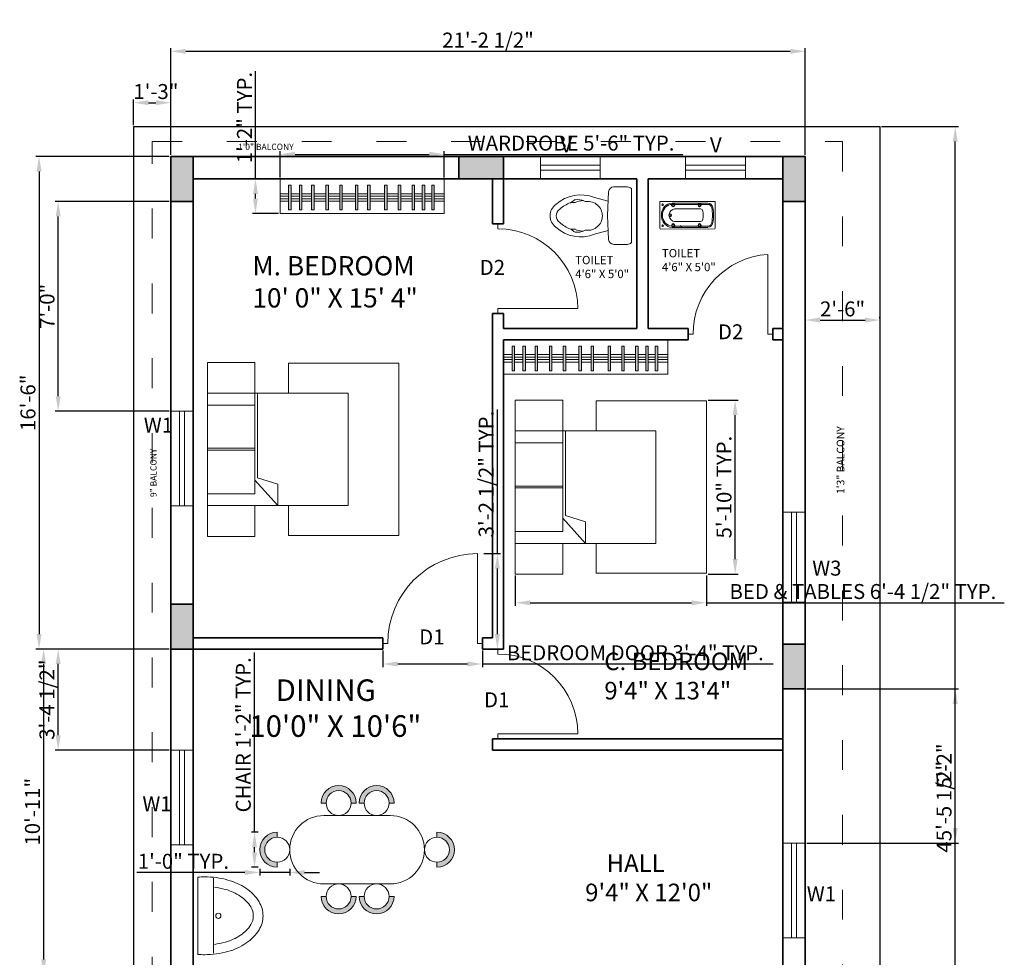
# Model space of a CAD drawing. Units: inches. Extents: x 40559 to 41508, y 131086 to 132358.
# Tile 2 of 5: x 40559 to 40954, y 131334 to 131710. Entities that reach past the tile are written whole.
import ezdxf

# ---------------------------------------------------------------- set-up
doc = ezdxf.new("R2010")
doc.units = ezdxf.units.IN
doc.linetypes.add('ACAD_ISO03W100', pattern=[30, 12, -18])
for name, color, linetype, lineweight in [('A-ANNO-DIMS', 2, 'Continuous', 18), ('A-ANNO-TEXT', 7, 'Continuous', 18), ('A-AREA-IDEN', 7, 'Continuous', 18), ('A-FLOR-FIXT', 4, 'Continuous', 18), ('A-FLOR-OVHD', 240, 'ACAD_ISO03W100', 13), ('A-FURN', 9, 'Continuous', 18), ('A-FURN-PATT', 252, 'Continuous', 13), ('A-WALL', 7, 'Continuous', 35), ('C-PROP', 7, 'Continuous', 25), ('Doors', 50, 'Continuous', 18), ('Windows', 70, 'Continuous', 18)]:
    doc.layers.add(name, color=color, linetype=linetype, lineweight=lineweight)
doc.layers.add('A-COLS', color=177, linetype='Continuous', lineweight=35, true_color=0x293189)
doc.styles.get("Standard").update_dxf_attribs({"font": 'arial.ttf'})
doc.dimstyles.new('ISO-25', dxfattribs={"dimtxt": 6, "dimasz": 6, "dimexe": 1.25, "dimexo": 0.625, "dimtad": 1, "dimdec": 0, "dimlunit": 3, "dimtxsty": 'Standard', "dimcen": 2.5, "dimclrd": 1, "dimclre": 1, "dimclrt": 2, "dimadec": 0, "dimazin": 0, "dimtfac": 1, "dimtdec": 0, "dimtmove": 0, "dimatfit": 3, "dimfxl": 1, "dimarcsym": 0})

# ---------------------------------------------------------------- blocks, each defined once
blk = doc.blocks.new('*D8')
at = {"layer": 'A-ANNO-DIMS', "color": 0, "lineweight": -2, "transparency": 16777216}
for p, q in [((40604.44, 131667.98), (40604.44, 131678.2)), ((40610.44, 131676.95), (40613.44, 131676.95)), ((40619.44, 131667.98), (40619.44, 131678.2))]:
    blk.add_line(p, q, dxfattribs=at)
at = {"layer": 'A-ANNO-DIMS', "color": 0, "transparency": 16777216}
for points in [[(40610.44, 131677.95), (40610.44, 131675.95), (40604.44, 131676.95)], [(40613.44, 131677.95), (40613.44, 131675.95), (40619.44, 131676.95)]]:
    blk.add_solid(points, dxfattribs=at)
at = {"layer": 'Defpoints', "color": 0, "transparency": 16777216}
for p in [(40619.44, 131676.95), (40604.44, 131667.35), (40619.44, 131667.35)]:
    blk.add_point(p, dxfattribs=at)
at = {"layer": 'A-ANNO-DIMS', "color": 0, "transparency": 16777216, "insert": (40613.44, 131680.64), "char_height": 6, "attachment_point": 5}
blk.add_mtext('1\'-3"', dxfattribs=at)
blk = doc.blocks.new('*D9')
at = {"layer": 'A-ANNO-DIMS', "color": 0, "lineweight": -2, "transparency": 16777216}
for p, q in [((40618.81, 131655.35), (40565.32, 131655.35)), ((40566.57, 131649.35), (40566.57, 131463.85)), ((40618.81, 131457.85), (40565.32, 131457.85))]:
    blk.add_line(p, q, dxfattribs=at)
at = {"layer": 'A-ANNO-DIMS', "color": 0, "transparency": 16777216}
for points in [[(40565.57, 131649.35), (40567.57, 131649.35), (40566.57, 131655.35)], [(40565.57, 131463.85), (40567.57, 131463.85), (40566.57, 131457.85)]]:
    blk.add_solid(points, dxfattribs=at)
at = {"layer": 'Defpoints', "color": 0, "transparency": 16777216}
for p in [(40619.44, 131655.35), (40566.57, 131457.85), (40619.44, 131457.85)]:
    blk.add_point(p, dxfattribs=at)
at = {"layer": 'A-ANNO-DIMS', "color": 0, "transparency": 16777216, "insert": (40562.88, 131556.6), "char_height": 6, "attachment_point": 5, "rotation": 90}
blk.add_mtext('16\'-6"', dxfattribs=at)
blk = doc.blocks.new('*D10')
at = {"layer": 'A-ANNO-DIMS', "color": 0, "lineweight": -2, "transparency": 16777216}
for p, q in [((40618.81, 131457.85), (40567.14, 131457.85)), ((40568.39, 131451.85), (40568.39, 131333.35)), ((40627.81, 131327.35), (40567.14, 131327.35))]:
    blk.add_line(p, q, dxfattribs=at)
at = {"layer": 'A-ANNO-DIMS', "color": 0, "transparency": 16777216}
for points in [[(40567.39, 131451.85), (40569.39, 131451.85), (40568.39, 131457.85)], [(40567.39, 131333.35), (40569.39, 131333.35), (40568.39, 131327.35)]]:
    blk.add_solid(points, dxfattribs=at)
at = {"layer": 'Defpoints', "color": 0, "transparency": 16777216}
for p in [(40619.44, 131457.85), (40568.39, 131327.35), (40628.44, 131327.35)]:
    blk.add_point(p, dxfattribs=at)
at = {"layer": 'A-ANNO-DIMS', "color": 0, "transparency": 16777216, "insert": (40564.7, 131392.6), "char_height": 6, "attachment_point": 5, "rotation": 90}
blk.add_mtext('10\'-11"', dxfattribs=at)
blk = doc.blocks.new('*D7')
at = {"layer": 'A-ANNO-DIMS', "color": 0, "lineweight": -2, "transparency": 16777216}
for p, q in [((40873.94, 131590.4), (40873.94, 131591.03)), ((40879.94, 131589.78), (40897.94, 131589.78)), ((40903.94, 131590.4), (40903.94, 131591.03))]:
    blk.add_line(p, q, dxfattribs=at)
at = {"layer": 'A-ANNO-DIMS', "color": 0, "transparency": 16777216}
for points in [[(40879.94, 131590.78), (40879.94, 131588.78), (40873.94, 131589.78)], [(40897.94, 131590.78), (40897.94, 131588.78), (40903.94, 131589.78)]]:
    blk.add_solid(points, dxfattribs=at)
at = {"layer": 'Defpoints', "color": 0, "transparency": 16777216}
for p in [(40873.94, 131589.78), (40903.94, 131589.78), (40903.94, 131589.78)]:
    blk.add_point(p, dxfattribs=at)
at = {"layer": 'A-ANNO-DIMS', "color": 0, "transparency": 16777216, "insert": (40888.94, 131593.47), "char_height": 6, "attachment_point": 5}
blk.add_mtext('2\'-6"', dxfattribs=at)
blk = doc.blocks.new('WIN-36IN')
for p, q in [((0, 5.5), (36, 5.5)), ((0, 3.5), (36, 3.5))]:
    blk.add_line(p, q)
blk.add_lwpolyline([(0, 9), (36, 9), (36, 0), (0, 0)], close=True)
blk = doc.blocks.new('WIN-38IN')
for p, q in [((0, 5.5), (38, 5.5)), ((0, 3.5), (38, 3.5))]:
    blk.add_line(p, q)
blk.add_lwpolyline([(0, 9), (38, 9), (38, 0), (0, 0)], close=True)
blk = doc.blocks.new('VENT-24IN')
for p, q in [((0, 5.5), (24, 5.5)), ((0, 3.5), (24, 3.5))]:
    blk.add_line(p, q)
blk.add_lwpolyline([(0, 9), (24, 9), (24, 0), (0, 0)], close=True)
blk = doc.blocks.new('DOOR-INT-36IN')
for p, q in [((2.25, 34), (2.25, 36)), ((4.5, 0), (0, 0)), ((2.25, 0), (2.25, 2)), ((2.25, 2), (34.25, 2))]:
    blk.add_line(p, q)
blk.add_arc((2.25, 2), 32, 0, 90)
blk = doc.blocks.new('DOOR-BATH-34IN')
for p, q in [((32, 2.25), (32, 34.25)), ((34, 4.5), (34, 0)), ((0, 2.25), (2, 2.25)), ((34, 2.25), (32, 2.25))]:
    blk.add_line(p, q)
blk.add_arc((34.07, 2.25), 32.07, 93.6952, 180)
blk = doc.blocks.new('DOOR-INT-40IN')
for p, q in [((38, 2.25), (38, 38.25)), ((40, 4.5), (40, 0)), ((2, 2.25), (0, 2.25)), ((40, 2.25), (38, 2.25))]:
    blk.add_line(p, q)
blk.add_arc((38, 2.25), 36, 90, 180)
blk = doc.blocks.new('COL-9X18IN')
h = blk.add_hatch(color=256)
h.dxf.hatch_style = 1
h.paths.add_polyline_path([(9, 18), (0, 18), (0, 0), (9, 0)])
blk.add_lwpolyline([(0, 18), (9, 18), (9, 0), (0, 0)], close=True)
blk = doc.blocks.new('WARDROBE-PLAN')
h = blk.add_hatch(color=256)
h.dxf.hatch_style = 1
h.paths.add_polyline_path([(4.39, 11.35), (3.39, 11.35), (3.39, 1.43), (4.39, 1.43)])
h.paths.add_polyline_path([(19.37, 11.35), (18.37, 11.35), (18.37, 1.43), (19.37, 1.43)])
h.paths.add_polyline_path([(48.38, 11.35), (47.38, 11.35), (47.38, 1.43), (48.38, 1.43)])
h.paths.add_polyline_path([(61.87, 11.35), (60.87, 11.35), (60.87, 1.43), (61.87, 1.43)])
h = blk.add_hatch(color=256)
h.dxf.hatch_style = 1
h.paths.add_polyline_path([(8.74, 11.35), (7.74, 11.35), (7.74, 1.43), (8.74, 1.43)])
h.paths.add_polyline_path([(36.12, 11.35), (35.12, 11.35), (35.12, 1.43), (36.12, 1.43)])
h.paths.add_polyline_path([(58.05, 11.35), (57.05, 11.35), (57.05, 1.43), (58.05, 1.43)])
h = blk.add_hatch(color=256)
h.dxf.hatch_style = 1
h.paths.add_polyline_path([(13.65, 11.35), (12.65, 11.35), (12.65, 1.43), (13.65, 1.43)])
h.paths.add_polyline_path([(31.22, 11.35), (30.22, 11.35), (30.22, 1.43), (31.22, 1.43)])
h.paths.add_polyline_path([(53.97, 11.35), (52.97, 11.35), (52.97, 1.43), (53.97, 1.43)])
h = blk.add_hatch(color=256)
h.dxf.hatch_style = 1
h.paths.add_polyline_path([(24.95, 11.35), (23.95, 11.35), (23.95, 1.43), (24.95, 1.43)])
h.paths.add_polyline_path([(42.93, 11.35), (41.93, 11.35), (41.93, 1.43), (42.93, 1.43)])
for p, q in [((0, 13.83), (0, 0)), ((65.87, 0), (65.87, 13.83)), ((0, 7.92), (3.39, 7.92)), ((3.39, 11.35), (3.39, 1.43)), ((3.39, 11.35), (4.39, 11.35)), ((4.39, 11.35), (4.39, 1.43)), ((4.39, 7.92), (7.74, 7.92)), ((7.74, 11.35), (7.74, 1.43)), ((7.74, 11.35), (8.74, 11.35)), ((8.74, 11.35), (8.74, 1.43)), ((8.74, 7.92), (12.65, 7.92)), ((12.65, 11.35), (12.65, 1.43)), ((12.65, 11.35), (13.65, 11.35)), ((13.65, 11.35), (13.65, 1.43)), ((13.65, 7.92), (18.37, 7.92)), ((18.37, 11.35), (18.37, 1.43)), ((18.37, 11.35), (19.37, 11.35)), ((19.37, 11.35), (19.37, 1.43)), ((19.37, 7.92), (23.95, 7.92)), ((23.95, 11.35), (23.95, 1.43)), ((23.95, 11.35), (24.95, 11.35)), ((24.95, 11.35), (24.95, 1.43)), ((24.95, 7.92), (30.22, 7.92)), ((30.22, 11.35), (30.22, 1.43)), ((30.22, 11.35), (31.22, 11.35)), ((31.22, 11.35), (31.22, 1.43)), ((31.22, 7.92), (35.12, 7.92)), ((35.12, 11.35), (35.12, 1.43)), ((35.12, 11.35), (36.12, 11.35)), ((36.12, 11.35), (36.12, 1.43)), ((36.12, 7.92), (41.93, 7.92)), ((41.93, 11.35), (41.93, 1.43)), ((41.93, 11.35), (42.93, 11.35)), ((42.93, 11.35), (42.93, 1.43)), ((42.93, 7.92), (47.38, 7.92)), ((47.38, 11.35), (47.38, 1.43)), ((47.38, 11.35), (48.38, 11.35)), ((48.38, 11.35), (48.38, 1.43)), ((48.38, 7.92), (52.97, 7.92)), ((52.97, 11.35), (52.97, 1.43)), ((52.97, 11.35), (53.97, 11.35)), ((53.97, 11.35), (53.97, 1.43)), ((53.97, 7.92), (57.05, 7.92)), ((57.05, 11.35), (57.05, 1.43)), ((57.05, 11.35), (58.05, 11.35)), ((58.05, 11.35), (58.05, 1.43)), ((58.05, 7.92), (60.87, 7.92)), ((60.87, 11.35), (60.87, 1.43)), ((60.87, 11.35), (61.87, 11.35)), ((61.87, 11.35), (61.87, 1.43)), ((61.87, 7.92), (65.87, 7.92)), ((0, 6.92), (3.39, 6.92)), ((0, 5.92), (3.39, 5.92)), ((0, 4.92), (3.39, 4.92)), ((4.39, 6.92), (7.74, 6.92)), ((4.39, 5.92), (7.74, 5.92)), ((4.39, 4.92), (7.74, 4.92)), ((8.74, 6.92), (12.65, 6.92)), ((8.74, 5.92), (12.65, 5.92)), ((8.74, 4.92), (12.65, 4.92)), ((13.65, 6.92), (18.37, 6.92)), ((13.65, 5.92), (18.37, 5.92)), ((13.65, 4.92), (18.37, 4.92)), ((19.37, 6.92), (23.95, 6.92)), ((19.37, 5.92), (23.95, 5.92)), ((19.37, 4.92), (23.95, 4.92)), ((24.95, 6.92), (30.22, 6.92)), ((24.95, 5.92), (30.22, 5.92)), ((24.95, 4.92), (30.22, 4.92)), ((31.22, 6.92), (35.12, 6.92)), ((31.22, 5.92), (35.12, 5.92)), ((31.22, 4.92), (35.12, 4.92)), ((36.12, 6.92), (41.93, 6.92)), ((36.12, 5.92), (41.93, 5.92)), ((36.12, 4.92), (41.93, 4.92)), ((42.93, 6.92), (47.38, 6.92)), ((42.93, 5.92), (47.38, 5.92)), ((42.93, 4.92), (47.38, 4.92)), ((48.38, 6.92), (52.97, 6.92)), ((48.38, 5.92), (52.97, 5.92)), ((48.38, 4.92), (52.97, 4.92)), ((53.97, 6.92), (57.05, 6.92)), ((53.97, 5.92), (57.05, 5.92)), ((53.97, 4.92), (57.05, 4.92)), ((58.05, 6.92), (60.87, 6.92)), ((58.05, 5.92), (60.87, 5.92)), ((58.05, 4.92), (60.87, 4.92)), ((61.87, 6.92), (65.87, 6.92)), ((61.87, 5.92), (65.87, 5.92)), ((61.87, 4.92), (65.87, 4.92)), ((0, 0), (65.87, 0)), ((3.39, 1.43), (4.39, 1.43)), ((7.74, 1.43), (8.74, 1.43)), ((12.65, 1.43), (13.65, 1.43)), ((18.37, 1.43), (19.37, 1.43)), ((23.95, 1.43), (24.95, 1.43)), ((30.22, 1.43), (31.22, 1.43)), ((35.12, 1.43), (36.12, 1.43)), ((41.93, 1.43), (42.93, 1.43)), ((47.38, 1.43), (48.38, 1.43)), ((52.97, 1.43), (53.97, 1.43)), ((57.05, 1.43), (58.05, 1.43)), ((60.87, 1.43), (61.87, 1.43))]:
    blk.add_line(p, q)
blk = doc.blocks.new('BED-WITH-SIDE-TABLES')
for p, q in [((0, 57.45), (0, 69.77)), ((0, 69.77), (19.02, 69.77)), ((19.02, 69.77), (19.02, 57.45)), ((32.44, 57.45), (32.44, 69.45)), ((32.44, 69.45), (76.71, 69.45)), ((76.71, 69.45), (76.71, 0.32)), ((0, 52.63), (0, 57.45)), ((0, 57.45), (56.44, 57.45)), ((19.02, 57.45), (19.02, 22.47)), ((20.12, 23.47), (20.12, 57.45)), ((56.44, 57.45), (56.44, 12.32)), ((0, 52.63), (19.02, 52.63)), ((0, 17.11), (0, 52.63)), ((19.02, 52.63), (19.02, 17.11)), ((0, 35.3), (19.02, 35.3)), ((0, 34.61), (19.02, 34.61)), ((19.02, 22.47), (28.22, 12.32)), ((28.22, 20.94), (20.12, 23.47)), ((28.22, 12.32), (28.22, 20.94)), ((0, 17.11), (19.02, 17.11)), ((0, 17.11), (0, 12.32)), ((0, 12.32), (56.44, 12.32)), ((0, 12.32), (0, 0)), ((19.02, 0), (19.02, 12.32)), ((32.44, 12.32), (32.44, 0.32)), ((0, 0), (19.02, 0)), ((32.44, 0.32), (76.71, 0.32))]:
    blk.add_line(p, q)
blk = doc.blocks.new('DINING-CHAIR')
for p, q in [((1.99, 5.01), (0, 5.01)), ((12.01, 5.01), (13.99, 5.01))]:
    blk.add_line(p, q)
blk.add_circle((7, 5.01), 5.01)
blk.add_arc((7, 5.01), 7, 0, 180)
blk = doc.blocks.new('*D48')
at = {"layer": 'A-ANNO-DIMS', "color": 1, "lineweight": -2, "transparency": 16777216}
for p, q in [((40704.44, 131457.23), (40704.44, 131450.6)), ((40744.44, 131457.23), (40744.44, 131450.6)), ((40710.44, 131451.85), (40738.44, 131451.85)), ((40744.44, 131451.85), (40861.11, 131451.85))]:
    blk.add_line(p, q, dxfattribs=at)
at = {"layer": 'A-ANNO-DIMS', "color": 1, "transparency": 16777216}
for points in [[(40710.44, 131452.85), (40710.44, 131450.85), (40704.44, 131451.85)], [(40738.44, 131452.85), (40738.44, 131450.85), (40744.44, 131451.85)]]:
    blk.add_solid(points, dxfattribs=at)
at = {"layer": 'Defpoints', "color": 0, "transparency": 16777216}
for p in [(40704.44, 131457.85), (40744.44, 131457.85), (40744.44, 131451.85)]:
    blk.add_point(p, dxfattribs=at)
at = {"layer": 'A-ANNO-DIMS', "color": 2, "transparency": 16777216, "insert": (40805.77, 131455.58), "char_height": 6, "attachment_point": 5}
blk.add_mtext('BEDROOM DOOR 3\'-4" TYP.', dxfattribs=at)
blk = doc.blocks.new('*D49')
at = {"layer": 'A-ANNO-DIMS', "color": 1, "lineweight": -2, "transparency": 16777216}
for p, q in [((40750.44, 131496.1), (40750.44, 131553.9)), ((40745.06, 131496.1), (40751.69, 131496.1)), ((40750.44, 131463.85), (40750.44, 131490.1)), ((40745.06, 131457.85), (40751.69, 131457.85))]:
    blk.add_line(p, q, dxfattribs=at)
at = {"layer": 'A-ANNO-DIMS', "color": 1, "transparency": 16777216}
for points in [[(40749.44, 131490.1), (40751.44, 131490.1), (40750.44, 131496.1)], [(40749.44, 131463.85), (40751.44, 131463.85), (40750.44, 131457.85)]]:
    blk.add_solid(points, dxfattribs=at)
at = {"layer": 'Defpoints', "color": 0, "transparency": 16777216}
for p in [(40744.44, 131496.1), (40750.44, 131496.1), (40744.44, 131457.85)]:
    blk.add_point(p, dxfattribs=at)
at = {"layer": 'A-ANNO-DIMS', "color": 2, "transparency": 16777216, "insert": (40746.71, 131528), "char_height": 6, "attachment_point": 5, "rotation": 90}
blk.add_mtext('3\'-2 1/2" TYP.', dxfattribs=at)
blk = doc.blocks.new('*D52')
at = {"layer": 'A-ANNO-DIMS', "color": 1, "lineweight": -2, "transparency": 16777216}
for p, q in [((40653.01, 131384.35), (40653.01, 131456.52)), ((40654.48, 131384.35), (40651.76, 131384.35)), ((40653.01, 131376.36), (40653.01, 131378.35)), ((40654.48, 131370.36), (40651.76, 131370.36))]:
    blk.add_line(p, q, dxfattribs=at)
at = {"layer": 'A-ANNO-DIMS', "color": 1, "transparency": 16777216}
for points in [[(40652.01, 131378.35), (40654.01, 131378.35), (40653.01, 131384.35)], [(40652.01, 131376.36), (40654.01, 131376.36), (40653.01, 131370.36)]]:
    blk.add_solid(points, dxfattribs=at)
at = {"layer": 'Defpoints', "color": 0, "transparency": 16777216}
for p in [(40653.01, 131384.35), (40655.11, 131384.35), (40655.11, 131370.36)]:
    blk.add_point(p, dxfattribs=at)
at = {"layer": 'A-ANNO-DIMS', "color": 2, "transparency": 16777216, "insert": (40649.28, 131423.44), "char_height": 6, "attachment_point": 5, "rotation": 90}
blk.add_mtext('CHAIR 1\'-2" TYP.', dxfattribs=at)
blk = doc.blocks.new('*D53')
at = {"layer": 'A-ANNO-DIMS', "color": 1, "lineweight": -2, "transparency": 16777216}
for p, q in [((40649.11, 131368.26), (40605.85, 131368.26)), ((40655.11, 131369.74), (40655.11, 131367.01)), ((40667.11, 131368.26), (40655.11, 131368.26)), ((40667.11, 131369.74), (40667.11, 131367.01)), ((40673.11, 131368.26), (40679.11, 131368.26))]:
    blk.add_line(p, q, dxfattribs=at)
at = {"layer": 'A-ANNO-DIMS', "color": 1, "transparency": 16777216}
for points in [[(40649.11, 131369.26), (40649.11, 131367.26), (40655.11, 131368.26)], [(40673.11, 131369.26), (40673.11, 131367.26), (40667.11, 131368.26)]]:
    blk.add_solid(points, dxfattribs=at)
at = {"layer": 'Defpoints', "color": 0, "transparency": 16777216}
for p in [(40655.11, 131370.36), (40655.11, 131368.26), (40667.11, 131370.36)]:
    blk.add_point(p, dxfattribs=at)
at = {"layer": 'A-ANNO-DIMS', "color": 2, "transparency": 16777216, "insert": (40624.48, 131371.95), "char_height": 6, "attachment_point": 5}
blk.add_mtext('1\'-0" TYP.', dxfattribs=at)
blk = doc.blocks.new('*D56')
at = {"layer": 'A-ANNO-DIMS', "color": 1, "lineweight": -2, "transparency": 16777216}
for p, q in [((40663.27, 131646.98), (40663.27, 131657.48)), ((40669.27, 131656.23), (40723.14, 131656.23)), ((40729.14, 131646.98), (40729.14, 131657.48)), ((40729.14, 131656.23), (40824.9, 131656.23))]:
    blk.add_line(p, q, dxfattribs=at)
at = {"layer": 'A-ANNO-DIMS', "color": 1, "transparency": 16777216}
for points in [[(40669.27, 131657.23), (40669.27, 131655.23), (40663.27, 131656.23)], [(40723.14, 131657.23), (40723.14, 131655.23), (40729.14, 131656.23)]]:
    blk.add_solid(points, dxfattribs=at)
at = {"layer": 'Defpoints', "color": 0, "transparency": 16777216}
for p in [(40729.14, 131656.23), (40663.27, 131646.35), (40729.14, 131646.35)]:
    blk.add_point(p, dxfattribs=at)
at = {"layer": 'A-ANNO-DIMS', "color": 2, "transparency": 16777216, "insert": (40780.02, 131659.96), "char_height": 6, "attachment_point": 5}
blk.add_mtext('WARDROBE 5\'-6" TYP.', dxfattribs=at)
blk = doc.blocks.new('*D57')
at = {"layer": 'A-ANNO-DIMS', "color": 1, "lineweight": -2, "transparency": 16777216}
for p, q in [((40653.39, 131646.35), (40653.39, 131689.61)), ((40662.64, 131646.35), (40652.14, 131646.35)), ((40653.39, 131638.52), (40653.39, 131640.35)), ((40662.64, 131632.52), (40652.14, 131632.52))]:
    blk.add_line(p, q, dxfattribs=at)
at = {"layer": 'A-ANNO-DIMS', "color": 1, "transparency": 16777216}
for points in [[(40652.39, 131640.35), (40654.39, 131640.35), (40653.39, 131646.35)], [(40652.39, 131638.52), (40654.39, 131638.52), (40653.39, 131632.52)]]:
    blk.add_solid(points, dxfattribs=at)
at = {"layer": 'Defpoints', "color": 0, "transparency": 16777216}
for p in [(40653.39, 131646.35), (40663.27, 131646.35), (40663.27, 131632.52)]:
    blk.add_point(p, dxfattribs=at)
at = {"layer": 'A-ANNO-DIMS', "color": 2, "transparency": 16777216, "insert": (40649.75, 131670.98), "char_height": 6, "attachment_point": 5, "rotation": 90}
blk.add_mtext('1\'-2" TYP.', dxfattribs=at)
blk = doc.blocks.new('*D58')
at = {"layer": 'A-ANNO-DIMS', "color": 1, "lineweight": -2, "transparency": 16777216}
for p, q in [((40757.62, 131487.28), (40757.62, 131475.15)), ((40834.33, 131487.28), (40834.33, 131475.15)), ((40763.62, 131476.4), (40828.33, 131476.4)), ((40834.33, 131476.4), (40953.83, 131476.4))]:
    blk.add_line(p, q, dxfattribs=at)
at = {"layer": 'A-ANNO-DIMS', "color": 1, "transparency": 16777216}
for points in [[(40763.62, 131477.4), (40763.62, 131475.4), (40757.62, 131476.4)], [(40828.33, 131477.4), (40828.33, 131475.4), (40834.33, 131476.4)]]:
    blk.add_solid(points, dxfattribs=at)
at = {"layer": 'Defpoints', "color": 0, "transparency": 16777216}
for p in [(40757.62, 131487.9), (40834.33, 131487.9), (40834.33, 131476.4)]:
    blk.add_point(p, dxfattribs=at)
at = {"layer": 'A-ANNO-DIMS', "color": 2, "transparency": 16777216, "insert": (40897.08, 131480.14), "char_height": 6, "attachment_point": 5}
blk.add_mtext('BED & TABLES 6\'-4 1/2" TYP.', dxfattribs=at)
blk = doc.blocks.new('*D59')
at = {"layer": 'A-ANNO-DIMS', "color": 1, "lineweight": -2, "transparency": 16777216}
for p, q in [((40834.96, 131557.68), (40847.09, 131557.68)), ((40845.84, 131493.9), (40845.84, 131551.68)), ((40834.96, 131487.9), (40847.09, 131487.9))]:
    blk.add_line(p, q, dxfattribs=at)
at = {"layer": 'A-ANNO-DIMS', "color": 1, "transparency": 16777216}
for points in [[(40844.84, 131551.68), (40846.84, 131551.68), (40845.84, 131557.68)], [(40844.84, 131493.9), (40846.84, 131493.9), (40845.84, 131487.9)]]:
    blk.add_solid(points, dxfattribs=at)
at = {"layer": 'Defpoints', "color": 0, "transparency": 16777216}
for p in [(40834.33, 131557.68), (40845.84, 131557.68), (40834.33, 131487.9)]:
    blk.add_point(p, dxfattribs=at)
at = {"layer": 'A-ANNO-DIMS', "color": 2, "transparency": 16777216, "insert": (40842.15, 131522.79), "char_height": 6, "attachment_point": 5, "rotation": 90}
blk.add_mtext('5\'-10" TYP.', dxfattribs=at)
blk = doc.blocks.new('*D65')
at = {"layer": 'A-ANNO-DIMS', "color": 1, "lineweight": -2, "transparency": 16777216}
for p, q in [((40904.56, 131667.35), (40935.39, 131667.35)), ((40934.14, 131127.85), (40934.14, 131661.35)), ((40904.56, 131121.85), (40935.39, 131121.85))]:
    blk.add_line(p, q, dxfattribs=at)
at = {"layer": 'A-ANNO-DIMS', "color": 1, "transparency": 16777216}
for points in [[(40933.14, 131661.35), (40935.14, 131661.35), (40934.14, 131667.35)], [(40933.14, 131127.85), (40935.14, 131127.85), (40934.14, 131121.85)]]:
    blk.add_solid(points, dxfattribs=at)
at = {"layer": 'Defpoints', "color": 0, "transparency": 16777216}
for p in [(40903.94, 131667.35), (40934.14, 131667.35), (40903.94, 131121.85)]:
    blk.add_point(p, dxfattribs=at)
at = {"layer": 'A-ANNO-DIMS', "color": 2, "transparency": 16777216, "insert": (40930.41, 131394.6), "char_height": 6, "attachment_point": 5, "rotation": 90}
blk.add_mtext('45\'-5 1/2"', dxfattribs=at)
blk = doc.blocks.new('*D66')
at = {"layer": 'A-ANNO-DIMS', "color": 1, "lineweight": -2, "transparency": 16777216}
for p, q in [((40619.44, 131655.98), (40619.44, 131698.8)), ((40625.44, 131697.55), (40867.94, 131697.55)), ((40873.94, 131655.98), (40873.94, 131698.8))]:
    blk.add_line(p, q, dxfattribs=at)
at = {"layer": 'A-ANNO-DIMS', "color": 1, "transparency": 16777216}
for points in [[(40625.44, 131698.55), (40625.44, 131696.55), (40619.44, 131697.55)], [(40867.94, 131698.55), (40867.94, 131696.55), (40873.94, 131697.55)]]:
    blk.add_solid(points, dxfattribs=at)
at = {"layer": 'Defpoints', "color": 0, "transparency": 16777216}
for p in [(40873.94, 131697.55), (40619.44, 131655.35), (40873.94, 131655.35)]:
    blk.add_point(p, dxfattribs=at)
at = {"layer": 'A-ANNO-DIMS', "color": 2, "transparency": 16777216, "insert": (40746.69, 131701.28), "char_height": 6, "attachment_point": 5}
blk.add_mtext('21\'-2 1/2"', dxfattribs=at)
blk = doc.blocks.new('*D67')
at = {"layer": 'A-ANNO-DIMS', "color": 1, "lineweight": -2, "transparency": 16777216}
for p, q in [((40618.81, 131457.85), (40572.99, 131457.85)), ((40574.24, 131423.3), (40574.24, 131451.85)), ((40618.81, 131417.3), (40572.99, 131417.3))]:
    blk.add_line(p, q, dxfattribs=at)
at = {"layer": 'A-ANNO-DIMS', "color": 1, "transparency": 16777216}
for points in [[(40573.24, 131451.85), (40575.24, 131451.85), (40574.24, 131457.85)], [(40573.24, 131423.3), (40575.24, 131423.3), (40574.24, 131417.3)]]:
    blk.add_solid(points, dxfattribs=at)
at = {"layer": 'Defpoints', "color": 0, "transparency": 16777216}
for p in [(40574.24, 131457.85), (40619.44, 131457.85), (40619.44, 131417.3)]:
    blk.add_point(p, dxfattribs=at)
at = {"layer": 'A-ANNO-DIMS', "color": 2, "transparency": 16777216, "insert": (40570.51, 131437.57), "char_height": 6, "attachment_point": 5, "rotation": 90}
blk.add_mtext('3\'-4 1/2"', dxfattribs=at)
blk = doc.blocks.new('*D68')
at = {"layer": 'A-ANNO-DIMS', "color": 1, "lineweight": -2, "transparency": 16777216}
for p, q in [((40618.81, 131637.35), (40572.99, 131637.35)), ((40574.24, 131559.22), (40574.24, 131631.35)), ((40618.81, 131553.22), (40572.99, 131553.22))]:
    blk.add_line(p, q, dxfattribs=at)
at = {"layer": 'A-ANNO-DIMS', "color": 1, "transparency": 16777216}
for points in [[(40573.24, 131631.35), (40575.24, 131631.35), (40574.24, 131637.35)], [(40573.24, 131559.22), (40575.24, 131559.22), (40574.24, 131553.22)]]:
    blk.add_solid(points, dxfattribs=at)
at = {"layer": 'Defpoints', "color": 0, "transparency": 16777216}
for p in [(40574.24, 131637.35), (40619.44, 131637.35), (40619.44, 131553.22)]:
    blk.add_point(p, dxfattribs=at)
at = {"layer": 'A-ANNO-DIMS', "color": 2, "transparency": 16777216, "insert": (40570.55, 131595.29), "char_height": 6, "attachment_point": 5, "rotation": 90}
blk.add_mtext('7\'-0"', dxfattribs=at)
blk = doc.blocks.new('*D69')
at = {"layer": 'A-ANNO-DIMS', "color": 1, "lineweight": -2, "transparency": 16777216}
for p, q in [((40874.56, 131441.85), (40935.39, 131441.85)), ((40934.14, 131386.06), (40934.14, 131435.85)), ((40874.56, 131380.06), (40935.39, 131380.06))]:
    blk.add_line(p, q, dxfattribs=at)
at = {"layer": 'A-ANNO-DIMS', "color": 1, "transparency": 16777216}
for points in [[(40933.14, 131435.85), (40935.14, 131435.85), (40934.14, 131441.85)], [(40933.14, 131386.06), (40935.14, 131386.06), (40934.14, 131380.06)]]:
    blk.add_solid(points, dxfattribs=at)
at = {"layer": 'Defpoints', "color": 0, "transparency": 16777216}
for p in [(40873.94, 131441.85), (40934.14, 131441.85), (40873.94, 131380.06)]:
    blk.add_point(p, dxfattribs=at)
at = {"layer": 'A-ANNO-DIMS', "color": 2, "transparency": 16777216, "insert": (40930.45, 131410.95), "char_height": 6, "attachment_point": 5, "rotation": 90}
blk.add_mtext('5\'-2"', dxfattribs=at)

msp = doc.modelspace()

# ---------------------------------------------------------------- hatches: boundary and pattern name
at = {"layer": 'A-FURN-PATT'}
h = msp.add_hatch(color=256, dxfattribs=at)
h.dxf.hatch_style = 1
h.paths.add_polyline_path([(40679.75, 131396.09), (40681.74, 131396.09, -1), (40691.75, 131396.09), (40693.74, 131396.09, 1)])
h.paths.add_polyline_path([(40694.98, 131396.09), (40696.97, 131396.09, -1), (40706.99, 131396.09), (40708.97, 131396.09, 1)])
h.paths.add_polyline_path([(40657.09, 131377.36, -0.414214), (40662.1, 131382.37), (40662.1, 131384.35, 1), (40662.1, 131370.36), (40662.1, 131372.35, -0.414214)])
h.paths.add_polyline_path([(40726.2, 131384.35), (40726.2, 131382.37, -0.414214), (40731.21, 131377.36, -0.414214), (40726.2, 131372.35), (40726.2, 131370.36, 1)])
h.paths.add_polyline_path([(40693.74, 131358.62), (40691.75, 131358.62, -1), (40681.74, 131358.62), (40679.75, 131358.62, 1)])
h.paths.add_polyline_path([(40708.97, 131358.62), (40706.99, 131358.62, -1), (40696.97, 131358.62), (40694.98, 131358.62, 1)])

# ---------------------------------------------------------------- linework, layer by layer
at = {"layer": 'A-FLOR-FIXT', "ltscale": 20}
for p, q in [((40794.64, 131631.65), (40795.07, 131641.2)), ((40802.62, 131643.17), (40797.13, 131643.17)), ((40804.32, 131621.03), (40804.32, 131642.27)), ((40780.19, 131636.9), (40781.61, 131636.9)), ((40780.38, 131637.12), (40781.14, 131637.77)), ((40794.9, 131637.44), (40789.38, 131638.94)), ((40794.64, 131631.65), (40795.07, 131622.1)), ((40780.19, 131626.21), (40781.61, 131626.21)), ((40780.38, 131625.99), (40781.14, 131625.34)), ((40794.91, 131625.68), (40789.38, 131624.17)), ((40802.62, 131620.13), (40797.13, 131620.13))]:
    msp.add_line(p, q, dxfattribs=at)
at = {"layer": 'A-FLOR-FIXT'}
for p, q in [((40815.57, 131637.2), (40815.57, 131626.44)), ((40815.57, 131637.2), (40815.57, 131626.44)), ((40837.69, 131637.35), (40815.7, 131637.35)), ((40837.69, 131637.35), (40815.7, 131637.35)), ((40820.54, 131636.69), (40834.93, 131636.69)), ((40820.54, 131636.17), (40834.93, 131636.17)), ((40837.82, 131626.45), (40837.82, 131637.21)), ((40837.82, 131626.45), (40837.82, 131637.21)), ((40821.56, 131634.33), (40831.98, 131634.33)), ((40831.98, 131629.32), (40821.56, 131629.32)), ((40815.7, 131626.29), (40837.69, 131626.3)), ((40815.7, 131626.29), (40837.69, 131626.3)), ((40834.93, 131627.48), (40820.54, 131627.47)), ((40834.93, 131626.96), (40820.54, 131626.96)), ((40630.27, 131335.38), (40630.27, 131366.38)), ((40636.52, 131335.84), (40636.52, 131365.92))]:
    msp.add_line(p, q, dxfattribs=at)
for points in [[(40656.43, 131350.88, 0.139889), (40654.83, 131356.49, 0.107118), (40649.58, 131361.92, 0.079812), (40642.34, 131365.22, 0.067459), (40633.02, 131366.49, 0.019694), (40630.27, 131366.38, 0.020439)], [(40652.53, 131350.88, 0.139889), (40651.52, 131354.43, 0.107118), (40647.41, 131358.67, 0.079812), (40641.3, 131361.46, 0.036069), (40636.91, 131362.34, 0.022172)], [(40630.27, 131335.38, 0.019694), (40633.02, 131335.27, 0.067459), (40642.34, 131336.53, 0.079812), (40649.58, 131339.84, 0.107118), (40654.83, 131345.27, 0.139889), (40656.43, 131350.88, 0.139889)], [(40636.91, 131339.42, 0.036069), (40641.3, 131340.3, 0.079812), (40647.41, 131343.09, 0.107118), (40651.52, 131347.33, 0.139889), (40652.53, 131350.88, 0.139889)]]:
    msp.add_lwpolyline(points, format="xyb", dxfattribs=at)
msp.add_circle((40638.49, 131350.88), 1.06, dxfattribs=at)
at = {"layer": 'A-FLOR-FIXT', "ltscale": 20}
for centre, radius, start, end in [((40783.9, 131625.25), 14.74, 68.2076, 132.5865), ((40797.13, 131641.11), 2.06, 90, 177.4245), ((40802.62, 131640.93), 2.24, 43.4731, 90), ((40804.03, 131642.27), 0.288, 0, 43.4731), ((40777.15, 131631.56), 5.57, 125.2885, 180), ((40783.9, 131625.25), 12.29, 109.6249, 133.388), ((40780.19, 131635.68), 1.23, 90, 109.6249), ((40779.59, 131638.06), 1.23, 288.6119, 310), ((40781.93, 131636.83), 1.23, 100.6032, 130), ((40784.86, 131630.32), 7.35, 89.5478, 116.498), ((40782.72, 131632.61), 5.51, 61.4258, 100.6032), ((40785.94, 131638.53), 1.23, 241.4258, 276.6477), ((40786.76, 131631.56), 5.8, 0, 96.6477), ((40777.15, 131631.56), 3.12, 122.7026, 180), ((40777.15, 131631.56), 5.57, 180, 234.7115), ((40777.15, 131631.56), 3.12, 180, 237.2974), ((40783.9, 131637.86), 12.29, 226.612, 250.3751), ((40786.76, 131631.56), 5.8, 263.3523, 0), ((40783.9, 131637.86), 14.74, 227.4135, 291.7924), ((40780.19, 131627.44), 1.23, 250.3751, 270), ((40779.59, 131625.05), 1.23, 50, 71.3881), ((40781.93, 131626.28), 1.23, 230, 259.3968), ((40784.86, 131632.79), 7.35, 243.502, 270.4522), ((40782.72, 131630.5), 5.51, 259.3968, 298.5742), ((40785.94, 131624.58), 1.23, 83.3523, 118.5742), ((40797.13, 131622.19), 2.06, 182.5755, 270), ((40802.62, 131622.37), 2.24, 270, 316.5269), ((40804.03, 131621.03), 0.288, 316.5269, 0)]:
    msp.add_arc(centre, radius, start, end, dxfattribs=at)
at = {"layer": 'A-FLOR-FIXT', "extrusion": (0, 0, -1)}
for centre, major_axis, start_param, end_param in [((40815.7, 131637.2), (0, 0.147), 4.712389, 6.283185), ((40815.7, 131637.2), (0, 0.147), 4.712389, 6.283185), ((40820.54, 131631.82), (0, 4.86), 3.141593, 6.283185), ((40816.74, 131636.02), (0, 0.324), 1.570796326794634, 7.85398163397422), ((40820.54, 131631.82), (0, 4.35), 3.141593, 6.283185), ((40821, 131635.91), (0, 0.737), 1.570796326794957, 7.853981633974544), ((40821, 131635.91), (0, 0.442), 1.570796326794643, 7.853981633974229), ((40831.6, 131635.92), (0, 0.737), 1.570796326794912, 7.853981633974498), ((40831.6, 131635.92), (0, 0.442), 1.57079632679489, 7.853981633974476), ((40834.93, 131634.41), (0, 2.28), 0, 1.388616), ((40834.93, 131634.41), (0, 1.77), 0, 1.388616), ((40837.69, 131637.21), (0, 0.147), 0, 1.570796), ((40837.69, 131637.21), (0, 0.147), 0, 1.570796), ((40819.76, 131631.82), (0, 0.59), 1.570796326794923, 7.853981633974509), ((40821.56, 131631.82), (0, 2.51), -1.413943, 0), ((40819.76, 131631.82), (0, 0.383), 1.570796326795266, 7.853981633974853), ((40831.98, 131633.26), (0, 1.07), 0, 1.388616), ((40825.05, 131631.82), (0, 9), 1.388616, 1.752977), ((40822.49, 131631.82), (0, 16.01), 1.388616, 1.752977), ((40822.49, 131631.82), (0, 16.52), 1.388616, 1.752977), ((40821.56, 131631.82), (0, 2.51), 3.141593, 4.555536), ((40821, 131627.73), (0, 0.737), 1.570796326794793, 7.853981633974379), ((40821, 131627.73), (0, 0.442), 1.570796326795149, 7.853981633974735), ((40831.6, 131627.73), (0, 0.737), 1.570796326795169, 7.853981633974756), ((40831.6, 131627.73), (0, 0.442), 1.570796326794995, 7.853981633974581), ((40831.98, 131630.39), (0, 1.07), 1.752977, 3.141593), ((40834.93, 131629.25), (0, 1.77), 1.752977, 3.141593), ((40834.93, 131629.25), (0, 2.28), 1.752977, 3.141593), ((40816.75, 131627.62), (0, 0.324), 1.570796326795611, 7.853981633975196), ((40824.69, 131627.73), (0, 0.841), 3.141593, 4.712389), ((40824.69, 131627.73), (0, 0.841), 3.141593, 4.712389)]:
    msp.add_ellipse(centre, major_axis=major_axis, ratio=0.888017, start_param=start_param, end_param=end_param, dxfattribs=at)
at = {"layer": 'A-FLOR-OVHD'}
for p, q in [((40611.94, 131202.46), (40611.94, 131661.35)), ((40611.94, 131661.35), (40888.94, 131661.35)), ((40888.94, 131661.35), (40888.94, 131121.85))]:
    msp.add_line(p, q, dxfattribs=at)
at = {"layer": 'A-FURN'}
for p, q in [((40680.84, 131391.08), (40707.46, 131391.08)), ((40680.84, 131363.63), (40707.46, 131363.63))]:
    msp.add_line(p, q, dxfattribs=at)
for centre, start, end in [((40680.84, 131377.36), 90, 270), ((40707.46, 131377.36), 270, 90)]:
    msp.add_arc(centre, 13.73, start, end, dxfattribs=at)
at = {"layer": 'A-WALL'}
for p, q in [((40619.44, 131655.35), (40619.44, 131198.35)), ((40619.44, 131655.35), (40873.94, 131655.35)), ((40873.94, 131655.35), (40873.94, 131264.35)), ((40628.44, 131646.35), (40628.44, 131207.35)), ((40628.44, 131646.35), (40748.44, 131646.35)), ((40628.44, 131646.35), (40748.44, 131646.35)), ((40748.44, 131646.35), (40748.44, 131628.35)), ((40752.94, 131646.35), (40752.94, 131628.35)), ((40752.94, 131646.35), (40806.44, 131646.35)), ((40752.94, 131646.35), (40806.44, 131646.35)), ((40806.44, 131646.35), (40806.44, 131586.35)), ((40810.94, 131646.35), (40864.94, 131646.35)), ((40810.94, 131646.35), (40810.94, 131586.35)), ((40810.94, 131646.35), (40864.94, 131646.35)), ((40864.94, 131646.35), (40864.94, 131273.35)), ((40864.94, 131646.35), (40864.94, 131586.35)), ((40748.44, 131628.35), (40752.94, 131628.35)), ((40748.44, 131592.35), (40748.44, 131462.35)), ((40752.94, 131592.35), (40748.44, 131592.35)), ((40752.94, 131592.35), (40752.94, 131586.35)), ((40752.94, 131586.35), (40806.44, 131586.35)), ((40810.94, 131586.35), (40826.94, 131586.35)), ((40826.94, 131586.35), (40826.94, 131581.85)), ((40860.94, 131586.35), (40864.94, 131586.35)), ((40860.94, 131586.35), (40860.94, 131581.85)), ((40752.94, 131581.85), (40752.94, 131457.85)), ((40752.94, 131581.85), (40826.94, 131581.85)), ((40860.94, 131581.85), (40864.94, 131581.85)), ((40628.44, 131462.35), (40704.44, 131462.35)), ((40704.44, 131462.35), (40704.44, 131457.85)), ((40744.44, 131462.35), (40748.44, 131462.35)), ((40744.44, 131462.35), (40744.44, 131457.85)), ((40628.44, 131457.85), (40704.44, 131457.85)), ((40744.44, 131457.85), (40748.44, 131457.85)), ((40748.44, 131457.85), (40752.94, 131457.85)), ((40748.44, 131421.85), (40748.44, 131417.35)), ((40748.44, 131421.85), (40864.94, 131421.85)), ((40748.44, 131417.35), (40864.94, 131417.35))]:
    msp.add_line(p, q, dxfattribs=at)
at = {"layer": 'C-PROP'}
for p, q in [((40604.44, 131667.35), (40604.44, 131121.85)), ((40604.44, 131667.35), (40903.94, 131667.35)), ((40903.94, 131667.35), (40903.94, 131121.85))]:
    msp.add_line(p, q, dxfattribs=at)

# ---------------------------------------------------------------- block references
at = {"layer": 'A-COLS'}
for p in [(40619.44, 131637.35), (40619.44, 131457.85)]:
    msp.add_blockref('COL-9X18IN', p, dxfattribs=at)
for p, rotation in [((40734.94, 131655.35), 270.0000000000411), ((40873.94, 131655.35), 180), ((40873.94, 131459.85), 180)]:
    msp.add_blockref('COL-9X18IN', p, dxfattribs=dict(at, rotation=rotation))
at = {"layer": 'A-FURN'}
for name, p in [('WARDROBE-PLAN', (40663.27, 131632.52)), ('WARDROBE-PLAN', (40752.94, 131568.02)), ('BED-WITH-SIDE-TABLES', (40634.15, 131503.04)), ('BED-WITH-SIDE-TABLES', (40757.62, 131487.9)), ('DINING-CHAIR', (40679.75, 131391.08)), ('DINING-CHAIR', (40694.98, 131391.08))]:
    msp.add_blockref(name, p, dxfattribs=at)
for p, rotation in [((40667.11, 131370.36), 90.00000000000003), ((40721.19, 131384.36), 270), ((40693.74, 131363.63), 180), ((40708.98, 131363.63), 180)]:
    msp.add_blockref('DINING-CHAIR', p, dxfattribs=dict(at, rotation=rotation))
at = {"layer": 'Doors'}
for name, p in [('DOOR-INT-36IN', (40748.44, 131592.35)), ('DOOR-BATH-34IN', (40826.94, 131581.85)), ('DOOR-INT-40IN', (40704.44, 131457.85)), ('DOOR-INT-36IN', (40748.44, 131421.85))]:
    msp.add_blockref(name, p, dxfattribs=at)
at = {"layer": 'Windows'}
for p in [(40767.69, 131646.35), (40825.94, 131646.35)]:
    msp.add_blockref('VENT-24IN', p, dxfattribs=at)
for name, p, rotation in [('WIN-38IN', (40619.44, 131553.22), 269.9999999999867), ('WIN-36IN', (40864.94, 131512.67), 269.9999999999951), ('WIN-38IN', (40619.44, 131417.3), 269.9999999999867), ('WIN-38IN', (40864.94, 131380.06), 269.9999999999867)]:
    msp.add_blockref(name, p, dxfattribs=dict(at, rotation=rotation))

# ---------------------------------------------------------------- texts
at = {"layer": 'A-ANNO-TEXT', "attachment_point": 1}
for s, width, insert, char_height in [('{\\fArial|b1|i0|c0|p34;1\'0" BALCONY}', 44.482, (40646.46, 131660.49), 2.5), ('{V}', 21.3561, (40775.73, 131663.06), 6), ('{V}', 21.3561, (40835.72, 131663.05), 6), ('{D2}', 6, (40743.35, 131613.89), 6), ('{D2}', 6, (40838.93, 131588.07), 6), ('{W1}', 21.3561, (40608.59, 131550.65), 6), ('{W3}', 21.3561, (40876.77, 131493.29), 6), ('{D1}', 6, (40719.06, 131465.71), 6), ('{D1}', 6, (40745.09, 131440.49), 6), ('{W1}', 21.3561, (40608.03, 131398.8), 6), ('{W1}', 21.3561, (40874.58, 131362.66), 6)]:
    msp.add_mtext_dynamic_manual_height_columns(s, width=width, gutter_width=12.5, heights=[0], dxfattribs=dict(at, insert=insert, char_height=char_height))
at = {"layer": 'A-ANNO-TEXT', "attachment_point": 1, "rotation": 90}
for s, width, gutter_width, insert, char_height in [('{\\fArial|b1|i0|c0|p34;1\'3" BALCONY}', 32.0122, 15.27, (40886.6, 131520), 3.0532), ('{\\fArial|b1|i0|c0|p34;9" BALCONY}', 44.482, 12.5, (40611.2, 131518.8), 2.5)]:
    msp.add_mtext_dynamic_manual_height_columns(s, width=width, gutter_width=gutter_width, heights=[0], dxfattribs=dict(at, insert=insert, char_height=char_height))
at = {"layer": 'A-AREA-IDEN', "attachment_point": 1}
for s, width, gutter_width, insert, char_height in [('{\\fArial|b1|i0|c0|p34;TOILET\\P4\'6" X 5\'0"}', 31.0377, 10.42, (40816.46, 131618.27), 3.3347), ('{\\fArial|b1|i0|c0|p34;M. BEDROOM\\P10\' 0" X 15\' 4"}', 78.1402, 16.09, (40652.14, 131615.41), 7.7236), ('{\\fArial|b1|i0|c0|p34;TOILET\\P4\'6" X 5\'0"}', 31.0494, 10.42, (40781.68, 131615.5), 3.3359), ('{\\fArial|b1|i0|c0|p34;C. BEDROOM\\P9\'4" X 13\'4"}', 75.8875, 14.66, (40793.35, 131456.42), 7.0382), ('{\\fArial|b1|i0|c0|p34;    DINING\\P10\'0" X 10\'6"}', 98.8896, 43.2, (40650.94, 131445.67), 8.639), ('{\\fArial|b1|i0|c0|p34;    HALL\\P9\'4" X 12\'0"}', 82.7784, 14.7, (40785.66, 131375.53), 7.0565)]:
    msp.add_mtext_dynamic_manual_height_columns(s, width=width, gutter_width=gutter_width, heights=[0], dxfattribs=dict(at, insert=insert, char_height=char_height))

# ---------------------------------------------------------------- dimensions: what is measured, and where the dimension line sits
at = {"layer": 'A-ANNO-DIMS'}
for base, p1, p2, override, picture, middle in [((40873.94, 131697.55), (40619.44, 131655.35), (40873.94, 131655.35), {"dimdec": 1, "dimlfac": 1, "dimrnd": 0, "dimzin": 1, "dimdsep": 46, "dimlunit": 4, "dimfrac": 2}, '*D66', (40746.69, 131701.28)), ((40903.94, 131589.78), (40873.94, 131589.78), (40903.94, 131589.78), {"dimclrd": 0, "dimclre": 0, "dimclrt": 0}, '*D7', (40888.94, 131593.47))]:
    dim = msp.add_linear_dim(base=base, p1=p1, p2=p2, dimstyle='ISO-25', override=override, dxfattribs=at)
    dim.commit()
    dim.dimension.update_dxf_attribs({"geometry": picture, "text_midpoint": middle})
for base, p1, p2, angle, text, picture, middle in [((40653.39, 131646.35), (40663.27, 131632.52), (40663.27, 131646.35), 90, '<> TYP.', '*D57', (40649.75, 131670.98)), ((40845.84, 131557.68), (40834.33, 131487.9), (40834.33, 131557.68), 90, '<> TYP.', '*D59', (40842.15, 131522.79)), ((40750.43804113, 131496.10041044), (40744.43804113, 131457.85041044), (40744.43804113, 131496.10041044), 90, '<> TYP.', '*D49', (40746.70867551, 131528.00030812)), ((40653.01, 131384.35), (40655.11, 131370.36), (40655.11, 131384.35), 90, 'CHAIR <> TYP.', '*D52', (40649.28, 131423.44)), ((40655.11, 131368.26), (40667.11, 131370.36), (40655.11, 131370.36), 180, '<> TYP.', '*D53', (40624.48, 131371.95))]:
    dim = msp.add_linear_dim(base=base, p1=p1, p2=p2, angle=angle, text=text, dimstyle='ISO-25', override={"dimdec": 1, "dimlfac": 1, "dimrnd": 0, "dimzin": 1, "dimdsep": 46, "dimlunit": 4, "dimfrac": 2}, dxfattribs=at)
    dim.commit()
    dim.dimension.update_dxf_attribs({"geometry": picture, "text_midpoint": middle})
dim = msp.add_linear_dim(base=(40619.44, 131676.95), p1=(40604.44, 131667.35), p2=(40619.44, 131667.35), dimstyle='ISO-25', override={"dimclrd": 0, "dimclre": 0, "dimclrt": 0}, dxfattribs=at)
dim.commit()
dim.dimension.update_dxf_attribs({"geometry": '*D8', "text_midpoint": (40613.44, 131676.95), "dimtype": 160})
for base, p1, p2, text, picture, middle in [((40729.14, 131656.23), (40663.27, 131646.35), (40729.14, 131646.35), 'WARDROBE <> TYP.', '*D56', (40780.02, 131659.96)), ((40834.33, 131476.4), (40757.62, 131487.9), (40834.33, 131487.9), 'BED & TABLES <> TYP.', '*D58', (40897.08, 131480.14)), ((40744.44, 131451.85), (40704.44, 131457.85), (40744.44, 131457.85), 'BEDROOM DOOR <> TYP.', '*D48', (40805.77, 131455.58))]:
    dim = msp.add_linear_dim(base=base, p1=p1, p2=p2, text=text, dimstyle='ISO-25', override={"dimdec": 1, "dimlfac": 1, "dimrnd": 0, "dimzin": 1, "dimdsep": 46, "dimlunit": 4, "dimfrac": 2}, dxfattribs=at)
    dim.commit()
    dim.dimension.update_dxf_attribs({"geometry": picture, "text_midpoint": middle})
for base, p1, p2, override, picture, middle in [((40934.14, 131667.35), (40903.94, 131121.85), (40903.94, 131667.35), {"dimdec": 1, "dimlfac": 1, "dimrnd": 0, "dimzin": 1, "dimdsep": 46, "dimlunit": 4, "dimfrac": 2}, '*D65', (40930.41, 131394.6)), ((40566.5716657, 131457.85041044), (40619.43804113, 131655.35041044), (40619.43804113, 131457.85041044), {"dimclrd": 0, "dimclre": 0, "dimclrt": 0}, '*D9', (40562.88322777, 131556.60041044)), ((40574.24, 131637.35), (40619.44, 131553.22), (40619.44, 131637.35), {"dimdec": 1, "dimlfac": 1, "dimrnd": 0, "dimzin": 1, "dimdsep": 46, "dimlunit": 4, "dimfrac": 2}, '*D68', (40570.55, 131595.29)), ((40568.38636267, 131327.35041044), (40619.43804113, 131457.85041044), (40628.43804113, 131327.35041044), {"dimclrd": 0, "dimclre": 0, "dimclrt": 0}, '*D10', (40564.69792474, 131392.60041044)), ((40574.238, 131457.8504), (40619.438, 131417.2953), (40619.438, 131457.8504), {"dimdec": 1, "dimlfac": 1, "dimrnd": 0, "dimzin": 1, "dimdsep": 46, "dimlunit": 4, "dimfrac": 2}, '*D67', (40570.5087, 131437.5729)), ((40934.14, 131441.85), (40873.94, 131380.06), (40873.94, 131441.85), {"dimdec": 1, "dimlfac": 1, "dimrnd": 0, "dimzin": 1, "dimdsep": 46, "dimlunit": 4, "dimfrac": 2}, '*D69', (40930.45, 131410.95))]:
    dim = msp.add_linear_dim(base=base, p1=p1, p2=p2, angle=90, dimstyle='ISO-25', override=override, dxfattribs=at)
    dim.commit()
    dim.dimension.update_dxf_attribs({"geometry": picture, "text_midpoint": middle})

doc.saveas('drawing.dxf')
